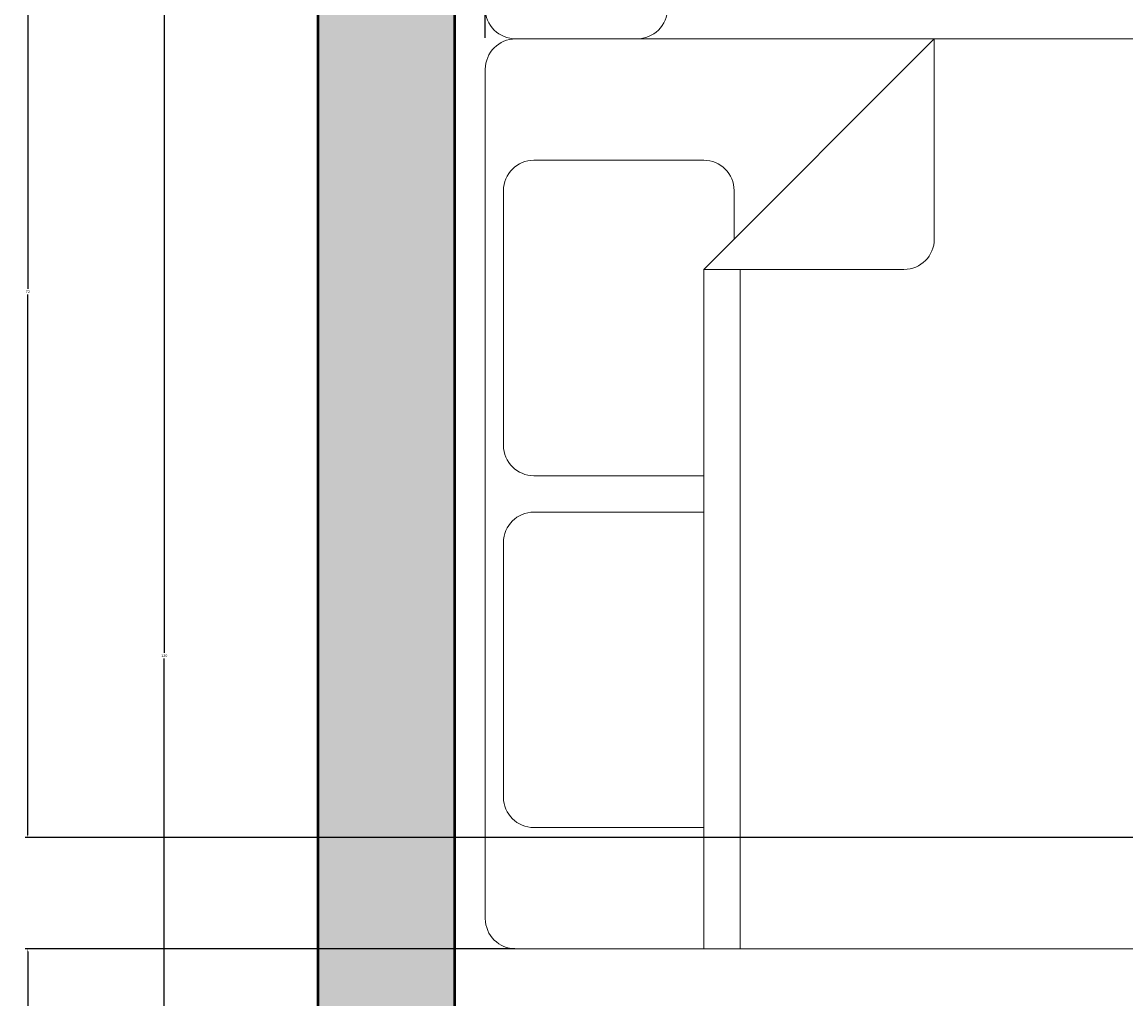
# Model space of a CAD drawing. Units: inches. Extents: x 2307 to 2544, y 2171 to 2540.
# Tile 22 of 52: x 2307 to 2380, y 2429 to 2493. Entities that reach past the tile are written whole.
import ezdxf

# ---------------------------------------------------------------- set-up
doc = ezdxf.new("R2010")
doc.units = ezdxf.units.IN
for name, color, linetype, lineweight in [('A-ANNO-DIMS', 2, 'Continuous', 18), ('A-FURN', 8, 'Continuous', 18), ('A-WALL', 7, 'Continuous', 50)]:
    doc.layers.add(name, color=color, linetype=linetype, lineweight=lineweight)
doc.layers.add('A-WALL-PATT', color=18, linetype='Continuous', lineweight=13, true_color=0x000000)
doc.styles.get("Standard").update_dxf_attribs({"font": 'arial.ttf'})
doc.dimstyles.get("Standard").update_dxf_attribs({"dimtxt": 0.18, "dimasz": 0.18, "dimexe": 0.18, "dimexo": 0.0625, "dimgap": 0.09, "dimtad": 0, "dimtih": 1, "dimtoh": 1, "dimdec": 4, "dimzin": 0, "dimdsep": 46, "dimtxsty": 'Standard', "dimcen": 0.09, "dimadec": 0, "dimazin": 0, "dimtfac": 1, "dimtdec": 4, "dimtofl": 0, "dimtmove": 0, "dimatfit": 3, "dimfxl": 1, "dimtolj": 1, "dimtzin": 0, "dimarcsym": 0})

# ---------------------------------------------------------------- blocks, each defined once
blk = doc.blocks.new('Bed - Queen')
for p, q in [((2, 0), (57.99999, 0)), ((9.99999, -1.2), (26.79998, -1.2)), ((33.19999, -1.2), (49.99999, -1.2)), ((0, -78.00003), (0, -2)), ((59.99999, -2), (59.99999, -78.00003)), ((7.99999, -14.4), (7.99999, -3.2)), ((28.79998, -3.2), (28.79998, -14.4)), ((31.19999, -14.4), (31.19999, -3.2)), ((51.99999, -3.2), (51.99999, -14.4)), ((0, -14.4), (44.8, -14.4)), ((59.99999, -29.6), (44.8, -14.4)), ((44.8, -14.4), (44.8, -27.6)), ((49.99999, -16.4), (46.79936, -16.4)), ((44.8, -16.8), (0, -16.8)), ((46.8, -29.6), (59.99999, -29.6))]:
    blk.add_line(p, q)
for centre, start, end in [((57.99999, -2), 0, 90), ((2, -2), 90, 180), ((9.99999, -3.2), 90, 180), ((26.79998, -3.2), 0, 90), ((33.19999, -3.2), 90, 180), ((49.99999, -3.2), 0, 90), ((49.99999, -14.4), 270, 0), ((46.8, -27.6), 180, 270)]:
    blk.add_arc(centre, 2, start, end)
blk = doc.blocks.new('*D26')
at = {"layer": 'A-ANNO-DIMS', "color": 0, "lineweight": -2, "transparency": 16777216}
for p, q in [((2337.708, 2492.237), (2337.708, 2504.354)), ((2337.888, 2504.174), (2376.714, 2504.174)), ((2417.528, 2504.174), (2378.702, 2504.174)), ((2417.708, 2492.237), (2417.708, 2504.354))]:
    blk.add_line(p, q, dxfattribs=at)
at = {"layer": 'A-ANNO-DIMS', "color": 0, "transparency": 16777216}
for points in [[(2337.888, 2504.204), (2337.888, 2504.144), (2337.708, 2504.174)], [(2417.528, 2504.204), (2417.528, 2504.144), (2417.708, 2504.174)]]:
    blk.add_solid(points, dxfattribs=at)
at = {"layer": 'Defpoints', "color": 0, "transparency": 16777216}
for p in [(2337.708, 2504.174), (2337.708, 2492.174), (2417.708, 2492.174)]:
    blk.add_point(p, dxfattribs=at)
at = {"layer": 'A-ANNO-DIMS', "color": 0, "transparency": 16777216, "insert": (2377.708, 2504.174), "char_height": 0.18, "attachment_point": 5}
blk.add_mtext('\\A1;QUEEN BED 80', dxfattribs=at)
blk = doc.blocks.new('*D47')
at = {"layer": 'A-ANNO-DIMS', "color": 0, "lineweight": -2, "transparency": 16777216}
for p, q in [((2335.633, 2511.51), (2316.366, 2511.51)), ((2316.546, 2511.33), (2316.546, 2451.691)), ((2316.546, 2391.69), (2316.546, 2451.328)), ((2335.633, 2391.51), (2316.366, 2391.51))]:
    blk.add_line(p, q, dxfattribs=at)
at = {"layer": 'A-ANNO-DIMS', "color": 0, "transparency": 16777216}
for points in [[(2316.516, 2511.33), (2316.576, 2511.33), (2316.546, 2511.51)], [(2316.516, 2391.69), (2316.576, 2391.69), (2316.546, 2391.51)]]:
    blk.add_solid(points, dxfattribs=at)
at = {"layer": 'Defpoints', "color": 0, "transparency": 16777216}
for p in [(2316.546, 2511.51), (2335.696, 2511.51), (2335.696, 2391.51)]:
    blk.add_point(p, dxfattribs=at)
at = {"layer": 'A-ANNO-DIMS', "color": 0, "transparency": 16777216, "insert": (2316.546, 2451.51), "char_height": 0.18, "attachment_point": 5}
blk.add_mtext('\\A1;120', dxfattribs=at)
blk = doc.blocks.new('*D48')
at = {"layer": 'A-ANNO-DIMS', "color": 0, "lineweight": -2, "transparency": 16777216}
for p, q in [((2455.633, 2511.51), (2307.366, 2511.51)), ((2307.546, 2511.33), (2307.546, 2475.69)), ((2307.546, 2439.69), (2307.546, 2475.329)), ((2455.633, 2439.51), (2307.366, 2439.51))]:
    blk.add_line(p, q, dxfattribs=at)
at = {"layer": 'A-ANNO-DIMS', "color": 0, "transparency": 16777216}
for points in [[(2307.516, 2511.33), (2307.576, 2511.33), (2307.546, 2511.51)], [(2307.516, 2439.69), (2307.576, 2439.69), (2307.546, 2439.51)]]:
    blk.add_solid(points, dxfattribs=at)
at = {"layer": 'Defpoints', "color": 0, "transparency": 16777216}
for p in [(2307.546, 2511.51), (2455.696, 2511.51), (2455.696, 2439.51)]:
    blk.add_point(p, dxfattribs=at)
at = {"layer": 'A-ANNO-DIMS', "color": 0, "transparency": 16777216, "insert": (2307.546, 2475.51), "char_height": 0.18, "attachment_point": 5}
blk.add_mtext('\\A1;72', dxfattribs=at)
blk = doc.blocks.new('*D67')
at = {"layer": 'A-ANNO-DIMS', "color": 0, "lineweight": -2, "transparency": 16777216}
for p, q in [((2339.646, 2432.174), (2307.366, 2432.174)), ((2307.546, 2431.994), (2307.546, 2421.024)), ((2307.546, 2409.69), (2307.546, 2420.66)), ((2335.633, 2409.51), (2307.366, 2409.51))]:
    blk.add_line(p, q, dxfattribs=at)
at = {"layer": 'A-ANNO-DIMS', "color": 0, "transparency": 16777216}
for points in [[(2307.516, 2431.994), (2307.576, 2431.994), (2307.546, 2432.174)], [(2307.516, 2409.69), (2307.576, 2409.69), (2307.546, 2409.51)]]:
    blk.add_solid(points, dxfattribs=at)
at = {"layer": 'Defpoints', "color": 0, "transparency": 16777216}
for p in [(2307.546, 2432.174), (2339.708, 2432.174), (2335.696, 2409.51)]:
    blk.add_point(p, dxfattribs=at)
at = {"layer": 'A-ANNO-DIMS', "color": 0, "transparency": 16777216, "insert": (2307.546, 2420.842), "char_height": 0.18, "attachment_point": 5}
blk.add_mtext('\\A1;22.665', dxfattribs=at)

msp = doc.modelspace()

# ---------------------------------------------------------------- hatches: boundary and pattern name
at = {"layer": 'A-WALL-PATT'}
h = msp.add_hatch(color=256, dxfattribs=at)
h.dxf.hatch_style = 1
h.paths.add_polyline_path([(2367.4028, 2520.5096), (2326.6958, 2520.5096), (2326.6958, 2355.3983), (2335.6958, 2355.3983), (2335.6958, 2387.5096), (2415.6958, 2387.5096), (2415.6958, 2391.5096), (2335.6958, 2391.5096), (2335.6958, 2409.5096), (2335.6958, 2511.5096), (2367.4028, 2511.5096)])

# ---------------------------------------------------------------- linework, layer by layer
at = {"layer": 'A-FURN'}
msp.add_lwpolyline([(2339.7083, 2492.1742), (2347.7083, 2492.1742, 0.4142136), (2349.7083, 2494.1742), (2349.7083, 2502.1742, 0.4142136), (2347.7083, 2504.1742), (2339.7083, 2504.1742, 0.4142136), (2337.7083, 2502.1742), (2337.7083, 2494.1742, 0.4142136)], format="xyb", close=True, dxfattribs=at)
at = {"layer": 'A-WALL'}
msp.add_line((2335.6958, 2391.5096), (2335.6958, 2511.5096), dxfattribs=at)
msp.add_lwpolyline([(2433.7832, 2190.5096), (2326.6958, 2190.5096), (2326.6958, 2520.5096), (2524.6958, 2520.5096), (2524.6958, 2190.5096), (2469.785, 2190.5096)], dxfattribs=at)

# ---------------------------------------------------------------- block references
at = {"layer": 'A-FURN', "rotation": 90}
msp.add_blockref('Bed - Queen', (2337.7083, 2432.1742), dxfattribs=at)

# ---------------------------------------------------------------- dimensions: what is measured, and where the dimension line sits
at = {"layer": 'A-ANNO-DIMS'}
for base, p1, p2, override, picture, middle in [((2307.5458, 2511.5096), (2455.6958, 2439.5096), (2455.6958, 2511.5096), {"dimdec": 0, "dimlfac": 1, "dimrnd": 0, "dimzin": 0, "dimdsep": 46, "dimlunit": 2}, '*D48', (2307.5458, 2475.5096)), ((2316.5458, 2511.5096), (2335.6958, 2391.5096), (2335.6958, 2511.5096), {"dimdec": 0, "dimlfac": 1, "dimrnd": 0, "dimzin": 0, "dimdsep": 46, "dimlunit": 2}, '*D47', (2316.5458, 2451.5096)), ((2307.5458, 2432.1742), (2335.6958, 2409.5096), (2339.7083, 2432.1742), {"dimdec": 3, "dimlfac": 1, "dimrnd": 0, "dimzin": 0, "dimdsep": 46, "dimlunit": 2}, '*D67', (2307.5458, 2420.8419))]:
    dim = msp.add_linear_dim(base=base, p1=p1, p2=p2, angle=90, dimstyle='Standard', override=override, dxfattribs=at)
    dim.commit()
    dim.dimension.update_dxf_attribs({"geometry": picture, "text_midpoint": middle})
dim = msp.add_linear_dim(base=(2337.7083, 2504.1742), p1=(2417.7084, 2492.1742), p2=(2337.7083, 2492.1742), angle=180, text='QUEEN BED <>', dimstyle='Standard', override={"dimdec": 0, "dimlfac": 1, "dimrnd": 0, "dimzin": 0, "dimdsep": 46, "dimlunit": 2}, dxfattribs=at)
dim.commit()
dim.dimension.update_dxf_attribs({"geometry": '*D26', "text_midpoint": (2377.7083, 2504.1742)})

doc.saveas('drawing.dxf')
